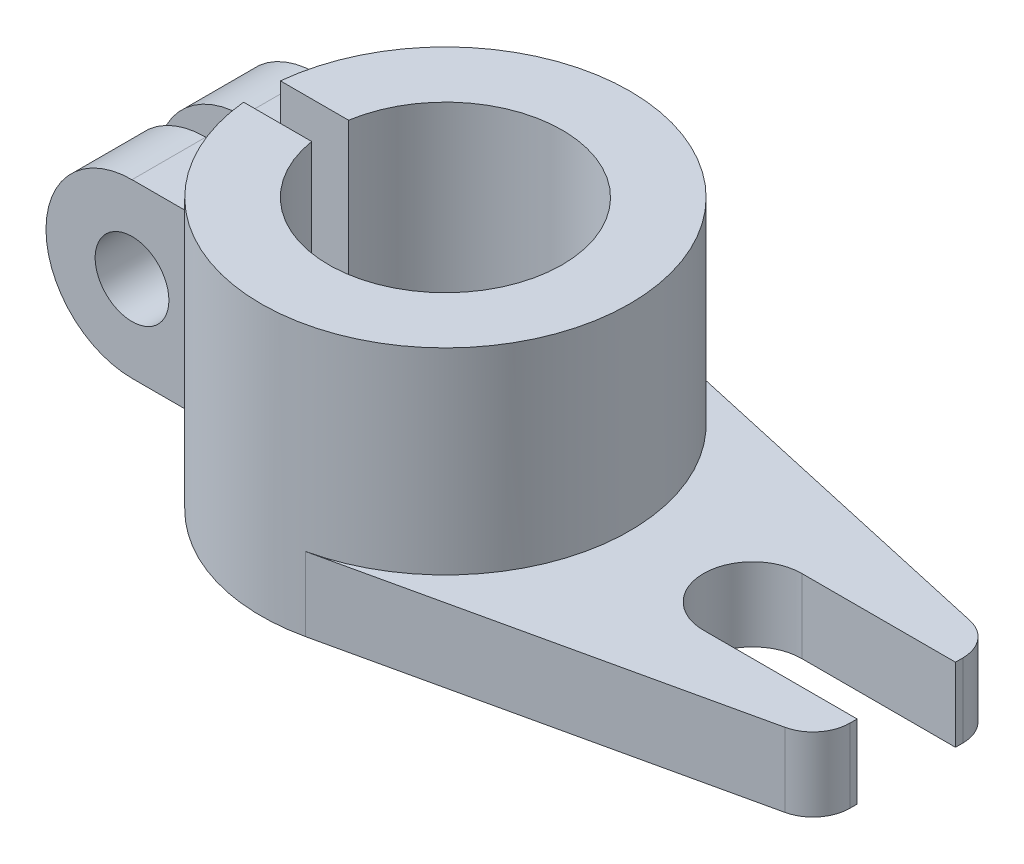
ISO-10303-21;
HEADER;
FILE_DESCRIPTION(('STEP AP214'),'2;1');
FILE_NAME('part.step','',(''),(''),'','','');
FILE_SCHEMA(('AUTOMOTIVE_DESIGN { 1 0 10303 214 1 1 1 1 }'));
ENDSEC;
DATA;
#1=APPLICATION_CONTEXT('core data for automotive mechanical design processes');
#2=APPLICATION_PROTOCOL_DEFINITION('international standard','automotive_design',2000,#1);
#3=PRODUCT_CONTEXT('',#1,'mechanical');
#4=PRODUCT('Part','Part','',(#3));
#5=PRODUCT_RELATED_PRODUCT_CATEGORY('part','',(#4));
#6=PRODUCT_DEFINITION_FORMATION('','',#4);
#7=PRODUCT_DEFINITION_CONTEXT('part definition',#1,'design');
#8=PRODUCT_DEFINITION('design','',#6,#7);
#9=PRODUCT_DEFINITION_SHAPE('','',#8);
#10=(LENGTH_UNIT() NAMED_UNIT(*) SI_UNIT(.MILLI.,.METRE.));
#11=(NAMED_UNIT(*) PLANE_ANGLE_UNIT() SI_UNIT($,.RADIAN.));
#12=(NAMED_UNIT(*) SI_UNIT($,.STERADIAN.) SOLID_ANGLE_UNIT());
#13=UNCERTAINTY_MEASURE_WITH_UNIT(LENGTH_MEASURE(1.E-05),#10,'distance_accuracy_value','');
#14=(GEOMETRIC_REPRESENTATION_CONTEXT(3) GLOBAL_UNCERTAINTY_ASSIGNED_CONTEXT((#13)) GLOBAL_UNIT_ASSIGNED_CONTEXT((#10,
#11,#12)) REPRESENTATION_CONTEXT('',''));
#15=CARTESIAN_POINT('',(0.,0.,0.));
#16=DIRECTION('',(0.,0.,1.));
#17=DIRECTION('',(1.,0.,0.));
#18=AXIS2_PLACEMENT_3D('',#15,#16,#17);
#19=CARTESIAN_POINT('',(0.,12.,0.));
#20=DIRECTION('',(0.,-1.,0.));
#21=DIRECTION('',(0.,0.,-1.));
#22=AXIS2_PLACEMENT_3D('',#19,#20,#21);
#23=CYLINDRICAL_SURFACE('',#22,30.);
#24=DIRECTION('',(0.,-1.,0.));
#25=VECTOR('',#24,1.);
#26=CARTESIAN_POINT('',(-25.9807621135332,12.,-15.));
#27=LINE('',#26,#25);
#28=CARTESIAN_POINT('',(-25.9807621135332,36.,-15.));
#29=VERTEX_POINT('',#28);
#30=CARTESIAN_POINT('',(-25.9807621135332,8.,-15.));
#31=VERTEX_POINT('',#30);
#32=EDGE_CURVE('E11',#29,#31,#27,.T.);
#33=ORIENTED_EDGE('',*,*,#32,.F.);
#34=CARTESIAN_POINT('',(0.,36.,0.));
#35=DIRECTION('',(0.,1.,0.));
#36=DIRECTION('',(0.,0.,1.));
#37=AXIS2_PLACEMENT_3D('',#34,#35,#36);
#38=CIRCLE('',#37,30.);
#39=CARTESIAN_POINT('',(-29.8496231131986,36.,-3.));
#40=VERTEX_POINT('',#39);
#41=EDGE_CURVE('E240',#29,#40,#38,.T.);
#42=ORIENTED_EDGE('',*,*,#41,.T.);
#43=DIRECTION('',(0.,-1.,0.));
#44=VECTOR('',#43,1.);
#45=CARTESIAN_POINT('',(-29.8496231131986,12.,-3.));
#46=LINE('',#45,#44);
#47=CARTESIAN_POINT('',(-29.8496231131986,44.,-3.));
#48=VERTEX_POINT('',#47);
#49=EDGE_CURVE('E386',#48,#40,#46,.T.);
#50=ORIENTED_EDGE('',*,*,#49,.F.);
#51=CARTESIAN_POINT('',(0.,44.,0.));
#52=DIRECTION('',(0.,1.,0.));
#53=DIRECTION('',(0.,0.,1.));
#54=AXIS2_PLACEMENT_3D('',#51,#52,#53);
#55=CIRCLE('',#54,30.);
#56=CARTESIAN_POINT('',(-29.8496231131986,44.,2.99999999999999));
#57=VERTEX_POINT('',#56);
#58=EDGE_CURVE('E274',#57,#48,#55,.T.);
#59=ORIENTED_EDGE('',*,*,#58,.F.);
#60=DIRECTION('',(0.,-1.,0.));
#61=VECTOR('',#60,1.);
#62=CARTESIAN_POINT('',(-29.8496231131986,12.,3.));
#63=LINE('',#62,#61);
#64=CARTESIAN_POINT('',(-29.8496231131986,36.,3.));
#65=VERTEX_POINT('',#64);
#66=EDGE_CURVE('E381',#57,#65,#63,.T.);
#67=ORIENTED_EDGE('',*,*,#66,.T.);
#68=CARTESIAN_POINT('',(0.,36.,0.));
#69=DIRECTION('',(0.,-1.,0.));
#70=DIRECTION('',(0.,0.,-1.));
#71=AXIS2_PLACEMENT_3D('',#68,#69,#70);
#72=CIRCLE('',#71,30.);
#73=CARTESIAN_POINT('',(-25.9807621135332,36.,15.));
#74=VERTEX_POINT('',#73);
#75=EDGE_CURVE('E283',#74,#65,#72,.T.);
#76=ORIENTED_EDGE('',*,*,#75,.F.);
#77=DIRECTION('',(0.,-1.,0.));
#78=VECTOR('',#77,1.);
#79=CARTESIAN_POINT('',(-25.9807621135332,12.,15.));
#80=LINE('',#79,#78);
#81=CARTESIAN_POINT('',(-25.9807621135332,8.,15.));
#82=VERTEX_POINT('',#81);
#83=EDGE_CURVE('E61',#74,#82,#80,.T.);
#84=ORIENTED_EDGE('',*,*,#83,.T.);
#85=CARTESIAN_POINT('',(0.,8.,0.));
#86=DIRECTION('',(0.,1.,0.));
#87=DIRECTION('',(0.,0.,1.));
#88=AXIS2_PLACEMENT_3D('',#85,#86,#87);
#89=CIRCLE('',#88,30.);
#90=CARTESIAN_POINT('',(-29.8496231131986,8.,3.));
#91=VERTEX_POINT('',#90);
#92=EDGE_CURVE('E47',#91,#82,#89,.T.);
#93=ORIENTED_EDGE('',*,*,#92,.F.);
#94=CARTESIAN_POINT('',(-29.8496231131986,0.,3.));
#95=VERTEX_POINT('',#94);
#96=EDGE_CURVE('E379',#91,#95,#63,.T.);
#97=ORIENTED_EDGE('',*,*,#96,.T.);
#98=CARTESIAN_POINT('',(0.,0.,0.));
#99=DIRECTION('',(0.,1.,0.));
#100=DIRECTION('',(0.,0.,1.));
#101=AXIS2_PLACEMENT_3D('',#98,#99,#100);
#102=CIRCLE('',#101,30.);
#103=CARTESIAN_POINT('',(6.5344558247283,0.,29.2797009389555));
#104=VERTEX_POINT('',#103);
#105=EDGE_CURVE('E339',#95,#104,#102,.T.);
#106=ORIENTED_EDGE('',*,*,#105,.T.);
#107=DIRECTION('',(0.,-1.,0.));
#108=VECTOR('',#107,1.);
#109=CARTESIAN_POINT('',(6.5344558247283,12.,29.2797009389555));
#110=LINE('',#109,#108);
#111=CARTESIAN_POINT('',(6.5344558247283,12.,29.2797009389555));
#112=VERTEX_POINT('',#111);
#113=EDGE_CURVE('E380',#112,#104,#110,.T.);
#114=ORIENTED_EDGE('',*,*,#113,.F.);
#115=CARTESIAN_POINT('',(0.,12.,0.));
#116=DIRECTION('',(0.,1.,0.));
#117=DIRECTION('',(0.,0.,1.));
#118=AXIS2_PLACEMENT_3D('',#115,#116,#117);
#119=CIRCLE('',#118,30.);
#120=CARTESIAN_POINT('',(6.5344558247283,12.,-29.2797009389555));
#121=VERTEX_POINT('',#120);
#122=EDGE_CURVE('E284',#112,#121,#119,.T.);
#123=ORIENTED_EDGE('',*,*,#122,.T.);
#124=DIRECTION('',(0.,-1.,0.));
#125=VECTOR('',#124,1.);
#126=CARTESIAN_POINT('',(6.5344558247283,12.,-29.2797009389555));
#127=LINE('',#126,#125);
#128=CARTESIAN_POINT('',(6.5344558247283,0.,-29.2797009389555));
#129=VERTEX_POINT('',#128);
#130=EDGE_CURVE('E288',#121,#129,#127,.T.);
#131=ORIENTED_EDGE('',*,*,#130,.T.);
#132=CARTESIAN_POINT('',(0.,0.,0.));
#133=DIRECTION('',(0.,1.,0.));
#134=DIRECTION('',(0.,0.,1.));
#135=AXIS2_PLACEMENT_3D('',#132,#133,#134);
#136=CIRCLE('',#135,30.);
#137=CARTESIAN_POINT('',(-29.8496231131986,0.,-3.));
#138=VERTEX_POINT('',#137);
#139=EDGE_CURVE('E326',#129,#138,#136,.T.);
#140=ORIENTED_EDGE('',*,*,#139,.T.);
#141=CARTESIAN_POINT('',(-29.8496231131986,8.,-3.));
#142=VERTEX_POINT('',#141);
#143=EDGE_CURVE('E389',#142,#138,#46,.T.);
#144=ORIENTED_EDGE('',*,*,#143,.F.);
#145=CARTESIAN_POINT('',(0.,8.,0.));
#146=DIRECTION('',(0.,-1.,0.));
#147=DIRECTION('',(0.,0.,-1.));
#148=AXIS2_PLACEMENT_3D('',#145,#146,#147);
#149=CIRCLE('',#148,30.);
#150=EDGE_CURVE('E232',#142,#31,#149,.T.);
#151=ORIENTED_EDGE('',*,*,#150,.T.);
#152=EDGE_LOOP('',(#33,#42,#50,#59,#67,#76,#84,#93,#97,#106,#114,#123,#131,#140,#144,#151));
#153=FACE_BOUND('',#152,.T.);
#154=ADVANCED_FACE('F41',(#153),#23,.T.);
#155=CARTESIAN_POINT('',(0.,12.,0.));
#156=DIRECTION('',(0.,1.,0.));
#157=DIRECTION('',(0.,0.,1.));
#158=AXIS2_PLACEMENT_3D('',#155,#156,#157);
#159=PLANE('',#158);
#160=DIRECTION('',(1.,0.,0.));
#161=VECTOR('',#160,1.);
#162=CARTESIAN_POINT('',(0.,12.,3.));
#163=LINE('',#162,#161);
#164=CARTESIAN_POINT('',(-18.7616630392937,12.,3.));
#165=VERTEX_POINT('',#164);
#166=CARTESIAN_POINT('',(0.,12.,3.));
#167=VERTEX_POINT('',#166);
#168=EDGE_CURVE('E305',#165,#167,#163,.T.);
#169=ORIENTED_EDGE('',*,*,#168,.F.);
#170=CARTESIAN_POINT('',(0.,12.,0.));
#171=DIRECTION('',(0.,1.,0.));
#172=DIRECTION('',(0.,0.,1.));
#173=AXIS2_PLACEMENT_3D('',#170,#171,#172);
#174=CIRCLE('',#173,19.);
#175=CARTESIAN_POINT('',(-18.7616630392937,12.,-3.));
#176=VERTEX_POINT('',#175);
#177=EDGE_CURVE('E268',#165,#176,#174,.T.);
#178=ORIENTED_EDGE('',*,*,#177,.T.);
#179=DIRECTION('',(1.,0.,0.));
#180=VECTOR('',#179,1.);
#181=CARTESIAN_POINT('',(0.,12.,-3.));
#182=LINE('',#181,#180);
#183=CARTESIAN_POINT('',(0.,12.,-3.));
#184=VERTEX_POINT('',#183);
#185=EDGE_CURVE('E297',#176,#184,#182,.T.);
#186=ORIENTED_EDGE('',*,*,#185,.T.);
#187=DIRECTION('',(0.,0.,1.));
#188=VECTOR('',#187,1.);
#189=CARTESIAN_POINT('',(0.,12.,0.));
#190=LINE('',#189,#188);
#191=EDGE_CURVE('E296',#184,#167,#190,.T.);
#192=ORIENTED_EDGE('',*,*,#191,.T.);
#193=EDGE_LOOP('',(#169,#178,#186,#192));
#194=FACE_BOUND('',#193,.T.);
#195=ADVANCED_FACE('F447',(#194),#159,.T.);
#196=CARTESIAN_POINT('',(6.5344558247283,12.,-29.2797009389555));
#197=DIRECTION('',(0.21781519415761,0.,-0.975990031298518));
#198=DIRECTION('',(-0.975990031298518,0.,-0.21781519415761));
#199=AXIS2_PLACEMENT_3D('',#196,#197,#198);
#200=PLANE('',#199);
#201=DIRECTION('',(0.975990031298518,0.,0.21781519415761));
#202=VECTOR('',#201,1.);
#203=CARTESIAN_POINT('',(6.5344558247283,0.,-29.2797009389555));
#204=LINE('',#203,#202);
#205=CARTESIAN_POINT('',(70.3068911649456,0.,-15.0473779232664));
#206=VERTEX_POINT('',#205);
#207=EDGE_CURVE('E295',#129,#206,#204,.T.);
#208=ORIENTED_EDGE('',*,*,#207,.F.);
#209=ORIENTED_EDGE('',*,*,#130,.F.);
#210=DIRECTION('',(0.975990031298518,0.,0.21781519415761));
#211=VECTOR('',#210,1.);
#212=CARTESIAN_POINT('',(6.5344558247283,12.,-29.2797009389555));
#213=LINE('',#212,#211);
#214=CARTESIAN_POINT('',(70.3068911649456,12.,-15.0473779232664));
#215=VERTEX_POINT('',#214);
#216=EDGE_CURVE('E291',#121,#215,#213,.T.);
#217=ORIENTED_EDGE('',*,*,#216,.T.);
#218=DIRECTION('',(0.,-1.,0.));
#219=VECTOR('',#218,1.);
#220=CARTESIAN_POINT('',(70.3068911649456,12.,-15.0473779232664));
#221=LINE('',#220,#219);
#222=EDGE_CURVE('E323',#215,#206,#221,.T.);
#223=ORIENTED_EDGE('',*,*,#222,.T.);
#224=EDGE_LOOP('',(#208,#209,#217,#223));
#225=FACE_BOUND('',#224,.T.);
#226=ADVANCED_FACE('F43',(#225),#200,.T.);
#227=CARTESIAN_POINT('',(0.,12.,-3.));
#228=DIRECTION('',(0.,0.,-1.));
#229=DIRECTION('',(-1.,0.,0.));
#230=AXIS2_PLACEMENT_3D('',#227,#228,#229);
#231=PLANE('',#230);
#232=ORIENTED_EDGE('',*,*,#49,.T.);
#233=DIRECTION('',(-1.,0.,0.));
#234=VECTOR('',#233,1.);
#235=CARTESIAN_POINT('',(-36.,36.,-3.));
#236=LINE('',#235,#234);
#237=CARTESIAN_POINT('',(-36.,36.,-3.));
#238=VERTEX_POINT('',#237);
#239=EDGE_CURVE('E225',#40,#238,#236,.T.);
#240=ORIENTED_EDGE('',*,*,#239,.T.);
#241=CARTESIAN_POINT('',(-36.,22.,-3.));
#242=DIRECTION('',(0.,0.,1.));
#243=DIRECTION('',(1.,0.,0.));
#244=AXIS2_PLACEMENT_3D('',#241,#242,#243);
#245=CIRCLE('',#244,14.);
#246=CARTESIAN_POINT('',(-36.,8.,-3.));
#247=VERTEX_POINT('',#246);
#248=EDGE_CURVE('E228',#238,#247,#245,.T.);
#249=ORIENTED_EDGE('',*,*,#248,.T.);
#250=DIRECTION('',(1.,0.,0.));
#251=VECTOR('',#250,1.);
#252=CARTESIAN_POINT('',(-25.,8.,-3.));
#253=LINE('',#252,#251);
#254=EDGE_CURVE('E57',#247,#142,#253,.T.);
#255=ORIENTED_EDGE('',*,*,#254,.T.);
#256=ORIENTED_EDGE('',*,*,#143,.T.);
#257=DIRECTION('',(1.,0.,0.));
#258=VECTOR('',#257,1.);
#259=CARTESIAN_POINT('',(0.,0.,-3.));
#260=LINE('',#259,#258);
#261=CARTESIAN_POINT('',(0.,0.,-3.));
#262=VERTEX_POINT('',#261);
#263=EDGE_CURVE('E328',#138,#262,#260,.T.);
#264=ORIENTED_EDGE('',*,*,#263,.T.);
#265=DIRECTION('',(0.,-1.,0.));
#266=VECTOR('',#265,1.);
#267=CARTESIAN_POINT('',(0.,12.,-3.));
#268=LINE('',#267,#266);
#269=EDGE_CURVE('E384',#184,#262,#268,.T.);
#270=ORIENTED_EDGE('',*,*,#269,.F.);
#271=ORIENTED_EDGE('',*,*,#185,.F.);
#272=DIRECTION('',(0.,-1.,0.));
#273=VECTOR('',#272,1.);
#274=CARTESIAN_POINT('',(-18.7616630392937,44.,-3.));
#275=LINE('',#274,#273);
#276=CARTESIAN_POINT('',(-18.7616630392937,44.,-3.));
#277=VERTEX_POINT('',#276);
#278=EDGE_CURVE('E278',#277,#176,#275,.T.);
#279=ORIENTED_EDGE('',*,*,#278,.F.);
#280=DIRECTION('',(1.,0.,0.));
#281=VECTOR('',#280,1.);
#282=CARTESIAN_POINT('',(0.,44.,-3.));
#283=LINE('',#282,#281);
#284=EDGE_CURVE('E279',#48,#277,#283,.T.);
#285=ORIENTED_EDGE('',*,*,#284,.F.);
#286=EDGE_LOOP('',(#232,#240,#249,#255,#256,#264,#270,#271,#279,#285));
#287=FACE_BOUND('',#286,.T.);
#288=CARTESIAN_POINT('',(-36.,22.,-3.));
#289=DIRECTION('',(0.,0.,1.));
#290=DIRECTION('',(1.,0.,0.));
#291=AXIS2_PLACEMENT_3D('',#288,#289,#290);
#292=CIRCLE('',#291,6.);
#293=CARTESIAN_POINT('',(-30.,22.,-3.));
#294=VERTEX_POINT('',#293);
#295=EDGE_CURVE('E227',#294,#294,#292,.T.);
#296=ORIENTED_EDGE('',*,*,#295,.F.);
#297=EDGE_LOOP('',(#296));
#298=FACE_BOUND('',#297,.T.);
#299=ADVANCED_FACE('F440',(#287,#298),#231,.F.);
#300=CARTESIAN_POINT('',(0.,12.,0.));
#301=DIRECTION('',(1.,0.,0.));
#302=DIRECTION('',(0.,0.,-1.));
#303=AXIS2_PLACEMENT_3D('',#300,#301,#302);
#304=PLANE('',#303);
#305=DIRECTION('',(0.,0.,1.));
#306=VECTOR('',#305,1.);
#307=CARTESIAN_POINT('',(0.,0.,0.));
#308=LINE('',#307,#306);
#309=CARTESIAN_POINT('',(0.,0.,3.));
#310=VERTEX_POINT('',#309);
#311=EDGE_CURVE('E332',#262,#310,#308,.T.);
#312=ORIENTED_EDGE('',*,*,#311,.T.);
#313=DIRECTION('',(0.,-1.,0.));
#314=VECTOR('',#313,1.);
#315=CARTESIAN_POINT('',(0.,12.,3.));
#316=LINE('',#315,#314);
#317=EDGE_CURVE('E382',#167,#310,#316,.T.);
#318=ORIENTED_EDGE('',*,*,#317,.F.);
#319=ORIENTED_EDGE('',*,*,#191,.F.);
#320=ORIENTED_EDGE('',*,*,#269,.T.);
#321=EDGE_LOOP('',(#312,#318,#319,#320));
#322=FACE_BOUND('',#321,.T.);
#323=ADVANCED_FACE('F444',(#322),#304,.F.);
#324=CARTESIAN_POINT('',(0.,12.,3.));
#325=DIRECTION('',(0.,0.,-1.));
#326=DIRECTION('',(-1.,0.,0.));
#327=AXIS2_PLACEMENT_3D('',#324,#325,#326);
#328=PLANE('',#327);
#329=ORIENTED_EDGE('',*,*,#96,.F.);
#330=DIRECTION('',(1.,0.,0.));
#331=VECTOR('',#330,1.);
#332=CARTESIAN_POINT('',(-25.,8.,3.));
#333=LINE('',#332,#331);
#334=CARTESIAN_POINT('',(-36.,8.,3.));
#335=VERTEX_POINT('',#334);
#336=EDGE_CURVE('E259',#335,#91,#333,.T.);
#337=ORIENTED_EDGE('',*,*,#336,.F.);
#338=CARTESIAN_POINT('',(-36.,22.,3.));
#339=DIRECTION('',(0.,0.,1.));
#340=DIRECTION('',(1.,0.,0.));
#341=AXIS2_PLACEMENT_3D('',#338,#339,#340);
#342=CIRCLE('',#341,14.);
#343=CARTESIAN_POINT('',(-36.,36.,3.));
#344=VERTEX_POINT('',#343);
#345=EDGE_CURVE('E241',#344,#335,#342,.T.);
#346=ORIENTED_EDGE('',*,*,#345,.F.);
#347=DIRECTION('',(-1.,0.,0.));
#348=VECTOR('',#347,1.);
#349=CARTESIAN_POINT('',(-36.,36.,3.));
#350=LINE('',#349,#348);
#351=EDGE_CURVE('E253',#65,#344,#350,.T.);
#352=ORIENTED_EDGE('',*,*,#351,.F.);
#353=ORIENTED_EDGE('',*,*,#66,.F.);
#354=DIRECTION('',(-1.,0.,0.));
#355=VECTOR('',#354,1.);
#356=CARTESIAN_POINT('',(0.,44.,3.));
#357=LINE('',#356,#355);
#358=CARTESIAN_POINT('',(-18.7616630392937,44.,3.));
#359=VERTEX_POINT('',#358);
#360=EDGE_CURVE('E275',#359,#57,#357,.T.);
#361=ORIENTED_EDGE('',*,*,#360,.F.);
#362=DIRECTION('',(0.,-1.,0.));
#363=VECTOR('',#362,1.);
#364=CARTESIAN_POINT('',(-18.7616630392937,44.,3.));
#365=LINE('',#364,#363);
#366=EDGE_CURVE('E287',#359,#165,#365,.T.);
#367=ORIENTED_EDGE('',*,*,#366,.T.);
#368=ORIENTED_EDGE('',*,*,#168,.T.);
#369=ORIENTED_EDGE('',*,*,#317,.T.);
#370=DIRECTION('',(1.,0.,0.));
#371=VECTOR('',#370,1.);
#372=CARTESIAN_POINT('',(0.,0.,3.));
#373=LINE('',#372,#371);
#374=EDGE_CURVE('E331',#95,#310,#373,.T.);
#375=ORIENTED_EDGE('',*,*,#374,.F.);
#376=EDGE_LOOP('',(#329,#337,#346,#352,#353,#361,#367,#368,#369,#375));
#377=FACE_BOUND('',#376,.T.);
#378=CARTESIAN_POINT('',(-36.,22.,3.));
#379=DIRECTION('',(0.,0.,1.));
#380=DIRECTION('',(1.,0.,0.));
#381=AXIS2_PLACEMENT_3D('',#378,#379,#380);
#382=CIRCLE('',#381,6.);
#383=CARTESIAN_POINT('',(-30.,22.,3.));
#384=VERTEX_POINT('',#383);
#385=EDGE_CURVE('E238',#384,#384,#382,.T.);
#386=ORIENTED_EDGE('',*,*,#385,.T.);
#387=EDGE_LOOP('',(#386));
#388=FACE_BOUND('',#387,.T.);
#389=ADVANCED_FACE('F406',(#377,#388),#328,.T.);
#390=CARTESIAN_POINT('',(6.5344558247283,12.,29.2797009389555));
#391=DIRECTION('',(-0.21781519415761,0.,-0.975990031298518));
#392=DIRECTION('',(-0.975990031298518,0.,0.21781519415761));
#393=AXIS2_PLACEMENT_3D('',#390,#391,#392);
#394=PLANE('',#393);
#395=DIRECTION('',(0.975990031298518,0.,-0.21781519415761));
#396=VECTOR('',#395,1.);
#397=CARTESIAN_POINT('',(6.5344558247283,0.,29.2797009389555));
#398=LINE('',#397,#396);
#399=CARTESIAN_POINT('',(70.3068911649456,0.,15.0473779232664));
#400=VERTEX_POINT('',#399);
#401=EDGE_CURVE('E336',#104,#400,#398,.T.);
#402=ORIENTED_EDGE('',*,*,#401,.T.);
#403=DIRECTION('',(0.,-1.,0.));
#404=VECTOR('',#403,1.);
#405=CARTESIAN_POINT('',(70.3068911649456,12.,15.0473779232664));
#406=LINE('',#405,#404);
#407=CARTESIAN_POINT('',(70.3068911649456,12.,15.0473779232664));
#408=VERTEX_POINT('',#407);
#409=EDGE_CURVE('E374',#408,#400,#406,.T.);
#410=ORIENTED_EDGE('',*,*,#409,.F.);
#411=DIRECTION('',(0.975990031298518,0.,-0.21781519415761));
#412=VECTOR('',#411,1.);
#413=CARTESIAN_POINT('',(6.5344558247283,12.,29.2797009389555));
#414=LINE('',#413,#412);
#415=EDGE_CURVE('E302',#112,#408,#414,.T.);
#416=ORIENTED_EDGE('',*,*,#415,.F.);
#417=ORIENTED_EDGE('',*,*,#113,.T.);
#418=EDGE_LOOP('',(#402,#410,#416,#417));
#419=FACE_BOUND('',#418,.T.);
#420=ADVANCED_FACE('F425',(#419),#394,.F.);
#421=CARTESIAN_POINT('',(69.,12.,9.19143773547529));
#422=DIRECTION('',(0.,-1.,0.));
#423=DIRECTION('',(0.,0.,-1.));
#424=AXIS2_PLACEMENT_3D('',#421,#422,#423);
#425=CYLINDRICAL_SURFACE('',#424,6.);
#426=CARTESIAN_POINT('',(69.,0.,9.19143773547529));
#427=DIRECTION('',(0.,1.,0.));
#428=DIRECTION('',(0.,0.,1.));
#429=AXIS2_PLACEMENT_3D('',#426,#427,#428);
#430=CIRCLE('',#429,6.);
#431=CARTESIAN_POINT('',(75.,0.,9.19143773547526));
#432=VERTEX_POINT('',#431);
#433=EDGE_CURVE('E345',#432,#400,#430,.F.);
#434=ORIENTED_EDGE('',*,*,#433,.F.);
#435=DIRECTION('',(0.,-1.,0.));
#436=VECTOR('',#435,1.);
#437=CARTESIAN_POINT('',(75.,12.,9.19143773547526));
#438=LINE('',#437,#436);
#439=CARTESIAN_POINT('',(75.,12.,9.19143773547526));
#440=VERTEX_POINT('',#439);
#441=EDGE_CURVE('E373',#440,#432,#438,.T.);
#442=ORIENTED_EDGE('',*,*,#441,.F.);
#443=CARTESIAN_POINT('',(69.,12.,9.19143773547529));
#444=DIRECTION('',(0.,1.,0.));
#445=DIRECTION('',(0.,0.,1.));
#446=AXIS2_PLACEMENT_3D('',#443,#444,#445);
#447=CIRCLE('',#446,6.);
#448=EDGE_CURVE('E308',#440,#408,#447,.F.);
#449=ORIENTED_EDGE('',*,*,#448,.T.);
#450=ORIENTED_EDGE('',*,*,#409,.T.);
#451=EDGE_LOOP('',(#434,#442,#449,#450));
#452=FACE_BOUND('',#451,.T.);
#453=ADVANCED_FACE('F496',(#452),#425,.T.);
#454=CARTESIAN_POINT('',(75.,12.,0.));
#455=DIRECTION('',(-1.,0.,0.));
#456=DIRECTION('',(0.,0.,1.));
#457=AXIS2_PLACEMENT_3D('',#454,#455,#456);
#458=PLANE('',#457);
#459=DIRECTION('',(0.,0.,-1.));
#460=VECTOR('',#459,1.);
#461=CARTESIAN_POINT('',(75.,0.,0.));
#462=LINE('',#461,#460);
#463=CARTESIAN_POINT('',(75.,0.,8.));
#464=VERTEX_POINT('',#463);
#465=EDGE_CURVE('E344',#432,#464,#462,.T.);
#466=ORIENTED_EDGE('',*,*,#465,.T.);
#467=DIRECTION('',(0.,-1.,0.));
#468=VECTOR('',#467,1.);
#469=CARTESIAN_POINT('',(75.,12.,8.));
#470=LINE('',#469,#468);
#471=CARTESIAN_POINT('',(75.,12.,8.));
#472=VERTEX_POINT('',#471);
#473=EDGE_CURVE('E371',#472,#464,#470,.T.);
#474=ORIENTED_EDGE('',*,*,#473,.F.);
#475=DIRECTION('',(0.,0.,-1.));
#476=VECTOR('',#475,1.);
#477=CARTESIAN_POINT('',(75.,12.,0.));
#478=LINE('',#477,#476);
#479=EDGE_CURVE('E310',#440,#472,#478,.T.);
#480=ORIENTED_EDGE('',*,*,#479,.F.);
#481=ORIENTED_EDGE('',*,*,#441,.T.);
#482=EDGE_LOOP('',(#466,#474,#480,#481));
#483=FACE_BOUND('',#482,.T.);
#484=ADVANCED_FACE('F640',(#483),#458,.F.);
#485=CARTESIAN_POINT('',(0.,12.,8.));
#486=DIRECTION('',(0.,0.,-1.));
#487=DIRECTION('',(-1.,0.,0.));
#488=AXIS2_PLACEMENT_3D('',#485,#486,#487);
#489=PLANE('',#488);
#490=DIRECTION('',(1.,0.,0.));
#491=VECTOR('',#490,1.);
#492=CARTESIAN_POINT('',(0.,0.,8.));
#493=LINE('',#492,#491);
#494=CARTESIAN_POINT('',(50.,0.,8.));
#495=VERTEX_POINT('',#494);
#496=EDGE_CURVE('E346',#495,#464,#493,.T.);
#497=ORIENTED_EDGE('',*,*,#496,.F.);
#498=DIRECTION('',(0.,-1.,0.));
#499=VECTOR('',#498,1.);
#500=CARTESIAN_POINT('',(50.,12.,8.));
#501=LINE('',#500,#499);
#502=CARTESIAN_POINT('',(50.,12.,8.));
#503=VERTEX_POINT('',#502);
#504=EDGE_CURVE('E369',#503,#495,#501,.T.);
#505=ORIENTED_EDGE('',*,*,#504,.F.);
#506=DIRECTION('',(1.,0.,0.));
#507=VECTOR('',#506,1.);
#508=CARTESIAN_POINT('',(0.,12.,8.));
#509=LINE('',#508,#507);
#510=EDGE_CURVE('E313',#503,#472,#509,.T.);
#511=ORIENTED_EDGE('',*,*,#510,.T.);
#512=ORIENTED_EDGE('',*,*,#473,.T.);
#513=EDGE_LOOP('',(#497,#505,#511,#512));
#514=FACE_BOUND('',#513,.T.);
#515=ADVANCED_FACE('F634',(#514),#489,.T.);
#516=CARTESIAN_POINT('',(50.,12.,0.));
#517=DIRECTION('',(0.,-1.,0.));
#518=DIRECTION('',(0.,0.,-1.));
#519=AXIS2_PLACEMENT_3D('',#516,#517,#518);
#520=CYLINDRICAL_SURFACE('',#519,8.);
#521=CARTESIAN_POINT('',(50.,0.,0.));
#522=DIRECTION('',(0.,1.,0.));
#523=DIRECTION('',(0.,0.,1.));
#524=AXIS2_PLACEMENT_3D('',#521,#522,#523);
#525=CIRCLE('',#524,8.);
#526=CARTESIAN_POINT('',(50.,0.,-8.));
#527=VERTEX_POINT('',#526);
#528=EDGE_CURVE('E352',#527,#495,#525,.T.);
#529=ORIENTED_EDGE('',*,*,#528,.F.);
#530=DIRECTION('',(0.,-1.,0.));
#531=VECTOR('',#530,1.);
#532=CARTESIAN_POINT('',(50.,12.,-8.));
#533=LINE('',#532,#531);
#534=CARTESIAN_POINT('',(50.,12.,-8.));
#535=VERTEX_POINT('',#534);
#536=EDGE_CURVE('E370',#535,#527,#533,.T.);
#537=ORIENTED_EDGE('',*,*,#536,.F.);
#538=CARTESIAN_POINT('',(50.,12.,0.));
#539=DIRECTION('',(0.,1.,0.));
#540=DIRECTION('',(0.,0.,1.));
#541=AXIS2_PLACEMENT_3D('',#538,#539,#540);
#542=CIRCLE('',#541,8.);
#543=EDGE_CURVE('E314',#535,#503,#542,.T.);
#544=ORIENTED_EDGE('',*,*,#543,.T.);
#545=ORIENTED_EDGE('',*,*,#504,.T.);
#546=EDGE_LOOP('',(#529,#537,#544,#545));
#547=FACE_BOUND('',#546,.T.);
#548=ADVANCED_FACE('F633',(#547),#520,.F.);
#549=CARTESIAN_POINT('',(0.,12.,-8.));
#550=DIRECTION('',(0.,0.,-1.));
#551=DIRECTION('',(-1.,0.,0.));
#552=AXIS2_PLACEMENT_3D('',#549,#550,#551);
#553=PLANE('',#552);
#554=DIRECTION('',(1.,0.,0.));
#555=VECTOR('',#554,1.);
#556=CARTESIAN_POINT('',(0.,0.,-8.));
#557=LINE('',#556,#555);
#558=CARTESIAN_POINT('',(75.,0.,-8.));
#559=VERTEX_POINT('',#558);
#560=EDGE_CURVE('E351',#527,#559,#557,.T.);
#561=ORIENTED_EDGE('',*,*,#560,.T.);
#562=DIRECTION('',(0.,-1.,0.));
#563=VECTOR('',#562,1.);
#564=CARTESIAN_POINT('',(75.,12.,-8.));
#565=LINE('',#564,#563);
#566=CARTESIAN_POINT('',(75.,12.,-8.));
#567=VERTEX_POINT('',#566);
#568=EDGE_CURVE('E365',#567,#559,#565,.T.);
#569=ORIENTED_EDGE('',*,*,#568,.F.);
#570=DIRECTION('',(1.,0.,0.));
#571=VECTOR('',#570,1.);
#572=CARTESIAN_POINT('',(0.,12.,-8.));
#573=LINE('',#572,#571);
#574=EDGE_CURVE('E320',#535,#567,#573,.T.);
#575=ORIENTED_EDGE('',*,*,#574,.F.);
#576=ORIENTED_EDGE('',*,*,#536,.T.);
#577=EDGE_LOOP('',(#561,#569,#575,#576));
#578=FACE_BOUND('',#577,.T.);
#579=ADVANCED_FACE('F629',(#578),#553,.F.);
#580=CARTESIAN_POINT('',(75.,12.,0.));
#581=DIRECTION('',(-1.,0.,0.));
#582=DIRECTION('',(0.,0.,1.));
#583=AXIS2_PLACEMENT_3D('',#580,#581,#582);
#584=PLANE('',#583);
#585=DIRECTION('',(0.,0.,-1.));
#586=VECTOR('',#585,1.);
#587=CARTESIAN_POINT('',(75.,0.,0.));
#588=LINE('',#587,#586);
#589=CARTESIAN_POINT('',(75.,0.,-9.19143773547526));
#590=VERTEX_POINT('',#589);
#591=EDGE_CURVE('E358',#559,#590,#588,.T.);
#592=ORIENTED_EDGE('',*,*,#591,.T.);
#593=DIRECTION('',(0.,-1.,0.));
#594=VECTOR('',#593,1.);
#595=CARTESIAN_POINT('',(75.,12.,-9.19143773547526));
#596=LINE('',#595,#594);
#597=CARTESIAN_POINT('',(75.,12.,-9.19143773547526));
#598=VERTEX_POINT('',#597);
#599=EDGE_CURVE('E363',#598,#590,#596,.T.);
#600=ORIENTED_EDGE('',*,*,#599,.F.);
#601=DIRECTION('',(0.,0.,-1.));
#602=VECTOR('',#601,1.);
#603=CARTESIAN_POINT('',(75.,12.,0.));
#604=LINE('',#603,#602);
#605=EDGE_CURVE('E317',#567,#598,#604,.T.);
#606=ORIENTED_EDGE('',*,*,#605,.F.);
#607=ORIENTED_EDGE('',*,*,#568,.T.);
#608=EDGE_LOOP('',(#592,#600,#606,#607));
#609=FACE_BOUND('',#608,.T.);
#610=ADVANCED_FACE('F621',(#609),#584,.F.);
#611=CARTESIAN_POINT('',(69.,12.,-9.19143773547529));
#612=DIRECTION('',(0.,-1.,0.));
#613=DIRECTION('',(0.,0.,-1.));
#614=AXIS2_PLACEMENT_3D('',#611,#612,#613);
#615=CYLINDRICAL_SURFACE('',#614,6.);
#616=CARTESIAN_POINT('',(69.,0.,-9.19143773547529));
#617=DIRECTION('',(0.,1.,0.));
#618=DIRECTION('',(0.,0.,1.));
#619=AXIS2_PLACEMENT_3D('',#616,#617,#618);
#620=CIRCLE('',#619,6.);
#621=EDGE_CURVE('E299',#590,#206,#620,.T.);
#622=ORIENTED_EDGE('',*,*,#621,.T.);
#623=ORIENTED_EDGE('',*,*,#222,.F.);
#624=CARTESIAN_POINT('',(69.,12.,-9.19143773547529));
#625=DIRECTION('',(0.,1.,0.));
#626=DIRECTION('',(0.,0.,1.));
#627=AXIS2_PLACEMENT_3D('',#624,#625,#626);
#628=CIRCLE('',#627,6.);
#629=EDGE_CURVE('E321',#598,#215,#628,.T.);
#630=ORIENTED_EDGE('',*,*,#629,.F.);
#631=ORIENTED_EDGE('',*,*,#599,.T.);
#632=EDGE_LOOP('',(#622,#623,#630,#631));
#633=FACE_BOUND('',#632,.T.);
#634=ADVANCED_FACE('F506',(#633),#615,.T.);
#635=ORIENTED_EDGE('',*,*,#122,.F.);
#636=ORIENTED_EDGE('',*,*,#415,.T.);
#637=ORIENTED_EDGE('',*,*,#448,.F.);
#638=ORIENTED_EDGE('',*,*,#479,.T.);
#639=ORIENTED_EDGE('',*,*,#510,.F.);
#640=ORIENTED_EDGE('',*,*,#543,.F.);
#641=ORIENTED_EDGE('',*,*,#574,.T.);
#642=ORIENTED_EDGE('',*,*,#605,.T.);
#643=ORIENTED_EDGE('',*,*,#629,.T.);
#644=ORIENTED_EDGE('',*,*,#216,.F.);
#645=EDGE_LOOP('',(#635,#636,#637,#638,#639,#640,#641,#642,#643,#644));
#646=FACE_BOUND('',#645,.T.);
#647=ADVANCED_FACE('F430',(#646),#159,.T.);
#648=CARTESIAN_POINT('',(0.,0.,0.));
#649=DIRECTION('',(0.,1.,0.));
#650=DIRECTION('',(0.,0.,1.));
#651=AXIS2_PLACEMENT_3D('',#648,#649,#650);
#652=PLANE('',#651);
#653=ORIENTED_EDGE('',*,*,#207,.T.);
#654=ORIENTED_EDGE('',*,*,#621,.F.);
#655=ORIENTED_EDGE('',*,*,#591,.F.);
#656=ORIENTED_EDGE('',*,*,#560,.F.);
#657=ORIENTED_EDGE('',*,*,#528,.T.);
#658=ORIENTED_EDGE('',*,*,#496,.T.);
#659=ORIENTED_EDGE('',*,*,#465,.F.);
#660=ORIENTED_EDGE('',*,*,#433,.T.);
#661=ORIENTED_EDGE('',*,*,#401,.F.);
#662=ORIENTED_EDGE('',*,*,#105,.F.);
#663=ORIENTED_EDGE('',*,*,#374,.T.);
#664=ORIENTED_EDGE('',*,*,#311,.F.);
#665=ORIENTED_EDGE('',*,*,#263,.F.);
#666=ORIENTED_EDGE('',*,*,#139,.F.);
#667=EDGE_LOOP('',(#653,#654,#655,#656,#657,#658,#659,#660,#661,#662,#663,#664,#665,#666));
#668=FACE_BOUND('',#667,.T.);
#669=ADVANCED_FACE('F418',(#668),#652,.F.);
#670=CARTESIAN_POINT('',(0.,44.,0.));
#671=DIRECTION('',(0.,-1.,0.));
#672=DIRECTION('',(0.,0.,-1.));
#673=AXIS2_PLACEMENT_3D('',#670,#671,#672);
#674=CYLINDRICAL_SURFACE('',#673,19.);
#675=ORIENTED_EDGE('',*,*,#177,.F.);
#676=ORIENTED_EDGE('',*,*,#366,.F.);
#677=CARTESIAN_POINT('',(0.,44.,0.));
#678=DIRECTION('',(0.,1.,0.));
#679=DIRECTION('',(0.,0.,1.));
#680=AXIS2_PLACEMENT_3D('',#677,#678,#679);
#681=CIRCLE('',#680,19.);
#682=EDGE_CURVE('E267',#359,#277,#681,.T.);
#683=ORIENTED_EDGE('',*,*,#682,.T.);
#684=ORIENTED_EDGE('',*,*,#278,.T.);
#685=EDGE_LOOP('',(#675,#676,#683,#684));
#686=FACE_BOUND('',#685,.T.);
#687=ADVANCED_FACE('F453',(#686),#674,.F.);
#688=CARTESIAN_POINT('',(0.,44.,0.));
#689=DIRECTION('',(0.,1.,0.));
#690=DIRECTION('',(0.,0.,1.));
#691=AXIS2_PLACEMENT_3D('',#688,#689,#690);
#692=PLANE('',#691);
#693=ORIENTED_EDGE('',*,*,#682,.F.);
#694=ORIENTED_EDGE('',*,*,#360,.T.);
#695=ORIENTED_EDGE('',*,*,#58,.T.);
#696=ORIENTED_EDGE('',*,*,#284,.T.);
#697=EDGE_LOOP('',(#693,#694,#695,#696));
#698=FACE_BOUND('',#697,.T.);
#699=ADVANCED_FACE('F454',(#698),#692,.T.);
#700=CARTESIAN_POINT('',(-36.,22.,15.));
#701=DIRECTION('',(0.,0.,1.));
#702=DIRECTION('',(1.,0.,0.));
#703=AXIS2_PLACEMENT_3D('',#700,#701,#702);
#704=PLANE('',#703);
#705=CARTESIAN_POINT('',(-36.,22.,15.));
#706=DIRECTION('',(0.,0.,1.));
#707=DIRECTION('',(1.,0.,0.));
#708=AXIS2_PLACEMENT_3D('',#705,#706,#707);
#709=CIRCLE('',#708,6.);
#710=CARTESIAN_POINT('',(-30.,22.,15.));
#711=VERTEX_POINT('',#710);
#712=EDGE_CURVE('E242',#711,#711,#709,.T.);
#713=ORIENTED_EDGE('',*,*,#712,.F.);
#714=EDGE_LOOP('',(#713));
#715=FACE_BOUND('',#714,.T.);
#716=ORIENTED_EDGE('',*,*,#83,.F.);
#717=DIRECTION('',(-1.,0.,0.));
#718=VECTOR('',#717,1.);
#719=CARTESIAN_POINT('',(-36.,36.,15.));
#720=LINE('',#719,#718);
#721=CARTESIAN_POINT('',(-36.,36.,15.));
#722=VERTEX_POINT('',#721);
#723=EDGE_CURVE('E255',#74,#722,#720,.T.);
#724=ORIENTED_EDGE('',*,*,#723,.T.);
#725=CARTESIAN_POINT('',(-36.,22.,15.));
#726=DIRECTION('',(0.,0.,1.));
#727=DIRECTION('',(1.,0.,0.));
#728=AXIS2_PLACEMENT_3D('',#725,#726,#727);
#729=CIRCLE('',#728,14.);
#730=CARTESIAN_POINT('',(-36.,8.,15.));
#731=VERTEX_POINT('',#730);
#732=EDGE_CURVE('E250',#722,#731,#729,.T.);
#733=ORIENTED_EDGE('',*,*,#732,.T.);
#734=DIRECTION('',(1.,0.,0.));
#735=VECTOR('',#734,1.);
#736=CARTESIAN_POINT('',(-25.,8.,15.));
#737=LINE('',#736,#735);
#738=EDGE_CURVE('E249',#731,#82,#737,.T.);
#739=ORIENTED_EDGE('',*,*,#738,.T.);
#740=EDGE_LOOP('',(#716,#724,#733,#739));
#741=FACE_BOUND('',#740,.T.);
#742=ADVANCED_FACE('F397',(#715,#741),#704,.T.);
#743=CARTESIAN_POINT('',(-36.,22.,15.));
#744=DIRECTION('',(0.,0.,-1.));
#745=DIRECTION('',(-1.,0.,0.));
#746=AXIS2_PLACEMENT_3D('',#743,#744,#745);
#747=CYLINDRICAL_SURFACE('',#746,14.);
#748=ORIENTED_EDGE('',*,*,#345,.T.);
#749=DIRECTION('',(0.,0.,-1.));
#750=VECTOR('',#749,1.);
#751=CARTESIAN_POINT('',(-36.,8.,15.));
#752=LINE('',#751,#750);
#753=EDGE_CURVE('E264',#731,#335,#752,.T.);
#754=ORIENTED_EDGE('',*,*,#753,.F.);
#755=ORIENTED_EDGE('',*,*,#732,.F.);
#756=DIRECTION('',(0.,0.,-1.));
#757=VECTOR('',#756,1.);
#758=CARTESIAN_POINT('',(-36.,36.,15.));
#759=LINE('',#758,#757);
#760=EDGE_CURVE('E258',#722,#344,#759,.T.);
#761=ORIENTED_EDGE('',*,*,#760,.T.);
#762=EDGE_LOOP('',(#748,#754,#755,#761));
#763=FACE_BOUND('',#762,.T.);
#764=ADVANCED_FACE('F403',(#763),#747,.T.);
#765=CARTESIAN_POINT('',(-25.,8.,15.));
#766=DIRECTION('',(0.,1.,0.));
#767=DIRECTION('',(0.,0.,1.));
#768=AXIS2_PLACEMENT_3D('',#765,#766,#767);
#769=PLANE('',#768);
#770=ORIENTED_EDGE('',*,*,#336,.T.);
#771=ORIENTED_EDGE('',*,*,#92,.T.);
#772=ORIENTED_EDGE('',*,*,#738,.F.);
#773=ORIENTED_EDGE('',*,*,#753,.T.);
#774=EDGE_LOOP('',(#770,#771,#772,#773));
#775=FACE_BOUND('',#774,.T.);
#776=ADVANCED_FACE('F398',(#775),#769,.F.);
#777=CARTESIAN_POINT('',(-36.,36.,15.));
#778=DIRECTION('',(0.,-1.,0.));
#779=DIRECTION('',(0.,0.,-1.));
#780=AXIS2_PLACEMENT_3D('',#777,#778,#779);
#781=PLANE('',#780);
#782=ORIENTED_EDGE('',*,*,#723,.F.);
#783=ORIENTED_EDGE('',*,*,#75,.T.);
#784=ORIENTED_EDGE('',*,*,#351,.T.);
#785=ORIENTED_EDGE('',*,*,#760,.F.);
#786=EDGE_LOOP('',(#782,#783,#784,#785));
#787=FACE_BOUND('',#786,.T.);
#788=ADVANCED_FACE('F554',(#787),#781,.F.);
#789=CARTESIAN_POINT('',(-36.,22.,15.));
#790=DIRECTION('',(0.,0.,-1.));
#791=DIRECTION('',(-1.,0.,0.));
#792=AXIS2_PLACEMENT_3D('',#789,#790,#791);
#793=CYLINDRICAL_SURFACE('',#792,6.);
#794=ORIENTED_EDGE('',*,*,#712,.T.);
#795=EDGE_LOOP('',(#794));
#796=FACE_BOUND('',#795,.T.);
#797=ORIENTED_EDGE('',*,*,#385,.F.);
#798=EDGE_LOOP('',(#797));
#799=FACE_BOUND('',#798,.T.);
#800=ADVANCED_FACE('F468',(#796,#799),#793,.F.);
#801=CARTESIAN_POINT('',(-36.,22.,-15.));
#802=DIRECTION('',(0.,0.,1.));
#803=DIRECTION('',(1.,0.,0.));
#804=AXIS2_PLACEMENT_3D('',#801,#802,#803);
#805=PLANE('',#804);
#806=CARTESIAN_POINT('',(-36.,22.,-15.));
#807=DIRECTION('',(0.,0.,1.));
#808=DIRECTION('',(1.,0.,0.));
#809=AXIS2_PLACEMENT_3D('',#806,#807,#808);
#810=CIRCLE('',#809,6.);
#811=CARTESIAN_POINT('',(-30.,22.,-15.));
#812=VERTEX_POINT('',#811);
#813=EDGE_CURVE('E235',#812,#812,#810,.T.);
#814=ORIENTED_EDGE('',*,*,#813,.T.);
#815=EDGE_LOOP('',(#814));
#816=FACE_BOUND('',#815,.T.);
#817=DIRECTION('',(-1.,0.,0.));
#818=VECTOR('',#817,1.);
#819=CARTESIAN_POINT('',(-36.,36.,-15.));
#820=LINE('',#819,#818);
#821=CARTESIAN_POINT('',(-36.,36.,-15.));
#822=VERTEX_POINT('',#821);
#823=EDGE_CURVE('E209',#29,#822,#820,.T.);
#824=ORIENTED_EDGE('',*,*,#823,.F.);
#825=ORIENTED_EDGE('',*,*,#32,.T.);
#826=DIRECTION('',(1.,0.,0.));
#827=VECTOR('',#826,1.);
#828=CARTESIAN_POINT('',(-25.,8.,-15.));
#829=LINE('',#828,#827);
#830=CARTESIAN_POINT('',(-36.,8.,-15.));
#831=VERTEX_POINT('',#830);
#832=EDGE_CURVE('E204',#831,#31,#829,.T.);
#833=ORIENTED_EDGE('',*,*,#832,.F.);
#834=CARTESIAN_POINT('',(-36.,22.,-15.));
#835=DIRECTION('',(0.,0.,1.));
#836=DIRECTION('',(1.,0.,0.));
#837=AXIS2_PLACEMENT_3D('',#834,#835,#836);
#838=CIRCLE('',#837,14.);
#839=EDGE_CURVE('E216',#822,#831,#838,.T.);
#840=ORIENTED_EDGE('',*,*,#839,.F.);
#841=EDGE_LOOP('',(#824,#825,#833,#840));
#842=FACE_BOUND('',#841,.T.);
#843=ADVANCED_FACE('F214',(#816,#842),#805,.F.);
#844=CARTESIAN_POINT('',(-36.,36.,-15.));
#845=DIRECTION('',(0.,1.,0.));
#846=DIRECTION('',(0.,0.,1.));
#847=AXIS2_PLACEMENT_3D('',#844,#845,#846);
#848=PLANE('',#847);
#849=ORIENTED_EDGE('',*,*,#41,.F.);
#850=ORIENTED_EDGE('',*,*,#823,.T.);
#851=DIRECTION('',(0.,0.,1.));
#852=VECTOR('',#851,1.);
#853=CARTESIAN_POINT('',(-36.,36.,-15.));
#854=LINE('',#853,#852);
#855=EDGE_CURVE('E207',#822,#238,#854,.T.);
#856=ORIENTED_EDGE('',*,*,#855,.T.);
#857=ORIENTED_EDGE('',*,*,#239,.F.);
#858=EDGE_LOOP('',(#849,#850,#856,#857));
#859=FACE_BOUND('',#858,.T.);
#860=ADVANCED_FACE('F456',(#859),#848,.T.);
#861=CARTESIAN_POINT('',(-25.,8.,-15.));
#862=DIRECTION('',(0.,-1.,0.));
#863=DIRECTION('',(0.,0.,-1.));
#864=AXIS2_PLACEMENT_3D('',#861,#862,#863);
#865=PLANE('',#864);
#866=ORIENTED_EDGE('',*,*,#150,.F.);
#867=ORIENTED_EDGE('',*,*,#254,.F.);
#868=DIRECTION('',(0.,0.,1.));
#869=VECTOR('',#868,1.);
#870=CARTESIAN_POINT('',(-36.,8.,-15.));
#871=LINE('',#870,#869);
#872=EDGE_CURVE('E203',#831,#247,#871,.T.);
#873=ORIENTED_EDGE('',*,*,#872,.F.);
#874=ORIENTED_EDGE('',*,*,#832,.T.);
#875=EDGE_LOOP('',(#866,#867,#873,#874));
#876=FACE_BOUND('',#875,.T.);
#877=ADVANCED_FACE('F201',(#876),#865,.T.);
#878=CARTESIAN_POINT('',(-36.,22.,-15.));
#879=DIRECTION('',(0.,0.,1.));
#880=DIRECTION('',(1.,0.,0.));
#881=AXIS2_PLACEMENT_3D('',#878,#879,#880);
#882=CYLINDRICAL_SURFACE('',#881,14.);
#883=ORIENTED_EDGE('',*,*,#248,.F.);
#884=ORIENTED_EDGE('',*,*,#855,.F.);
#885=ORIENTED_EDGE('',*,*,#839,.T.);
#886=ORIENTED_EDGE('',*,*,#872,.T.);
#887=EDGE_LOOP('',(#883,#884,#885,#886));
#888=FACE_BOUND('',#887,.T.);
#889=ADVANCED_FACE('F219',(#888),#882,.T.);
#890=CARTESIAN_POINT('',(-36.,22.,-15.));
#891=DIRECTION('',(0.,0.,1.));
#892=DIRECTION('',(1.,0.,0.));
#893=AXIS2_PLACEMENT_3D('',#890,#891,#892);
#894=CYLINDRICAL_SURFACE('',#893,6.);
#895=ORIENTED_EDGE('',*,*,#813,.F.);
#896=EDGE_LOOP('',(#895));
#897=FACE_BOUND('',#896,.T.);
#898=ORIENTED_EDGE('',*,*,#295,.T.);
#899=EDGE_LOOP('',(#898));
#900=FACE_BOUND('',#899,.T.);
#901=ADVANCED_FACE('F605',(#897,#900),#894,.F.);
#902=CLOSED_SHELL('',(#154,#195,#226,#299,#323,#389,#420,#453,#484,#515,#548,#579,#610,#634,
#647,#669,#687,#699,#742,#764,#776,#788,#800,#843,#860,#877,#889,#901));
#903=MANIFOLD_SOLID_BREP('B2',#902);
#904=ADVANCED_BREP_SHAPE_REPRESENTATION('',(#18,#903),#14);
#905=SHAPE_DEFINITION_REPRESENTATION(#9,#904);
ENDSEC;
END-ISO-10303-21;
